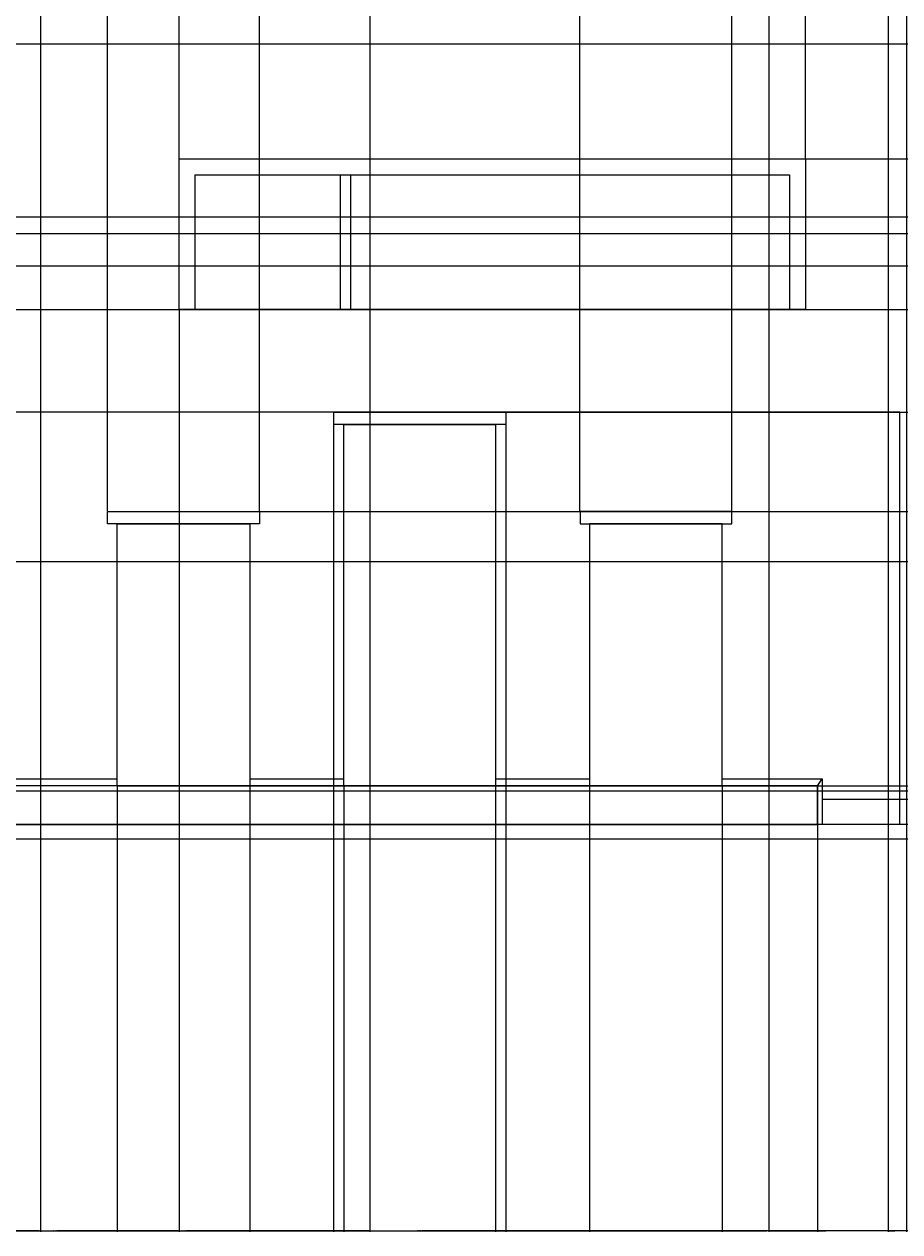
# Model space of a CAD drawing. Units: feet. Extents: x 2193 to 3502, y 890 to 1601.
# Tile 10 of 17: x 3145 to 3280, y 890 to 1076. Entities that reach past the tile are written whole.
import ezdxf

# ---------------------------------------------------------------- set-up
doc = ezdxf.new("R2010")
doc.units = ezdxf.units.FT
doc.layers.add('A-ANNO-DIMS', color=2, linetype='Continuous', lineweight=18)
doc.layers.add('A-ELEV', color=7, linetype='Continuous', lineweight=25)
doc.styles.get("Standard").update_dxf_attribs({"font": 'arial.ttf'})
doc.dimstyles.get("Standard").update_dxf_attribs({"dimtxt": 0.18, "dimasz": 0.18, "dimexe": 0.18, "dimexo": 0.0625, "dimgap": 0.09, "dimtad": 0, "dimtih": 1, "dimtoh": 1, "dimdec": 0, "dimzin": 0, "dimdsep": 46, "dimlunit": 3, "dimtxsty": 'Standard', "dimcen": 0.09, "dimadec": 0, "dimazin": 0, "dimtfac": 1, "dimtdec": 0, "dimtofl": 0, "dimtmove": 0, "dimatfit": 3, "dimfxl": 1, "dimtolj": 1, "dimtzin": 0, "dimarcsym": 0})

# ---------------------------------------------------------------- blocks, each defined once
blk = doc.blocks.new('*D13')
at = {"layer": 'A-ANNO-DIMS', "color": 0, "lineweight": -2, "transparency": 16777216}
for p, q in [((2934.37, 950.89), (2934.37, 1601.47)), ((2934.55, 1601.29), (3186.64, 1601.29)), ((3439.51, 1601.29), (3187.43, 1601.29)), ((3439.69, 1541.11), (3439.69, 1601.47))]:
    blk.add_line(p, q, dxfattribs=at)
at = {"layer": 'A-ANNO-DIMS', "color": 0, "transparency": 16777216}
for points in [[(2934.55, 1601.32), (2934.55, 1601.26), (2934.37, 1601.29)], [(3439.51, 1601.32), (3439.51, 1601.26), (3439.69, 1601.29)]]:
    blk.add_solid(points, dxfattribs=at)
at = {"layer": 'Defpoints', "color": 0, "transparency": 16777216}
for p in [(3439.69, 1601.29), (3439.69, 1541.04), (2934.37, 950.82)]:
    blk.add_point(p, dxfattribs=at)
at = {"layer": 'A-ANNO-DIMS', "color": 0, "transparency": 16777216, "insert": (3187.03, 1601.29), "char_height": 0.18, "attachment_point": 5}
blk.add_mtext('\\A1;505.3', dxfattribs=at)
blk = doc.blocks.new('*D16')
at = {"layer": 'A-ANNO-DIMS', "color": 0, "lineweight": -2, "transparency": 16777216}
for p, q in [((3132, 956.87), (3132, 890.39)), ((3305.41, 950.76), (3305.41, 890.39)), ((3132.18, 890.57), (3218.32, 890.57)), ((3305.23, 890.57), (3219.09, 890.57))]:
    blk.add_line(p, q, dxfattribs=at)
at = {"layer": 'A-ANNO-DIMS', "color": 0, "transparency": 16777216}
for points in [[(3132.18, 890.6), (3132.18, 890.54), (3132, 890.57)], [(3305.23, 890.6), (3305.23, 890.54), (3305.41, 890.57)]]:
    blk.add_solid(points, dxfattribs=at)
at = {"layer": 'Defpoints', "color": 0, "transparency": 16777216}
for p in [(3132, 956.94), (3305.41, 950.82), (3305.41, 890.57)]:
    blk.add_point(p, dxfattribs=at)
at = {"layer": 'A-ANNO-DIMS', "color": 0, "transparency": 16777216, "insert": (3218.71, 890.57), "char_height": 0.18, "attachment_point": 5}
blk.add_mtext('\\A1;173.4', dxfattribs=at)
blk = doc.blocks.new('*D25')
at = {"layer": 'A-ANNO-DIMS', "color": 0, "lineweight": -2, "transparency": 16777216}
for p, q in [((3070.17, 1073.03), (3501.85, 1073.03)), ((3501.67, 1072.85), (3501.67, 1056.13)), ((3501.67, 1039.05), (3501.67, 1055.77)), ((3067.73, 1038.87), (3501.85, 1038.87))]:
    blk.add_line(p, q, dxfattribs=at)
at = {"layer": 'A-ANNO-DIMS', "color": 0, "transparency": 16777216}
for points in [[(3501.64, 1072.85), (3501.7, 1072.85), (3501.67, 1073.03)], [(3501.64, 1039.05), (3501.7, 1039.05), (3501.67, 1038.87)]]:
    blk.add_solid(points, dxfattribs=at)
at = {"layer": 'Defpoints', "color": 0, "transparency": 16777216}
for p in [(3070.11, 1073.03), (3501.67, 1073.03), (3067.66, 1038.87)]:
    blk.add_point(p, dxfattribs=at)
at = {"layer": 'A-ANNO-DIMS', "color": 0, "transparency": 16777216, "insert": (3501.67, 1055.95), "char_height": 0.18, "attachment_point": 5}
blk.add_mtext('\\A1;34.165', dxfattribs=at)
blk = doc.blocks.new('*D31')
at = {"layer": 'A-ANNO-DIMS', "color": 0, "lineweight": -2, "transparency": 16777216}
for p, q in [((2760.54, 1541.04), (3501.85, 1541.04)), ((3501.67, 1540.86), (3501.67, 1246.12)), ((3501.67, 951), (3501.67, 1245.75)), ((2762.27, 950.82), (3501.85, 950.82))]:
    blk.add_line(p, q, dxfattribs=at)
at = {"layer": 'A-ANNO-DIMS', "color": 0, "transparency": 16777216}
for points in [[(3501.64, 1540.86), (3501.7, 1540.86), (3501.67, 1541.04)], [(3501.64, 951), (3501.7, 951), (3501.67, 950.82)]]:
    blk.add_solid(points, dxfattribs=at)
at = {"layer": 'Defpoints', "color": 0, "transparency": 16777216}
for p in [(2760.47, 1541.04), (3501.67, 1541.04), (2762.2, 950.82)]:
    blk.add_point(p, dxfattribs=at)
at = {"layer": 'A-ANNO-DIMS', "color": 0, "transparency": 16777216, "insert": (3501.67, 1245.93), "char_height": 0.18, "attachment_point": 5}
blk.add_mtext('\\A1;590.2', dxfattribs=at)
blk = doc.blocks.new('*D61')
at = {"layer": 'A-ANNO-DIMS', "color": 0, "lineweight": -2, "transparency": 16777216}
for p, q in [((2974.12, 1078.97), (2974.12, 890.39)), ((3147.5, 1078.97), (3147.5, 890.39)), ((2974.3, 890.57), (3060.42, 890.57)), ((3147.32, 890.57), (3061.19, 890.57))]:
    blk.add_line(p, q, dxfattribs=at)
at = {"layer": 'A-ANNO-DIMS', "color": 0, "transparency": 16777216}
for points in [[(2974.3, 890.6), (2974.3, 890.54), (2974.12, 890.57)], [(3147.32, 890.6), (3147.32, 890.54), (3147.5, 890.57)]]:
    blk.add_solid(points, dxfattribs=at)
at = {"layer": 'Defpoints', "color": 0, "transparency": 16777216}
for p in [(2974.12, 1079.03), (3147.5, 1079.03), (3147.5, 890.57)]:
    blk.add_point(p, dxfattribs=at)
at = {"layer": 'A-ANNO-DIMS', "color": 0, "transparency": 16777216, "insert": (3060.81, 890.57), "char_height": 0.18, "attachment_point": 5}
blk.add_mtext('\\A1;173.4', dxfattribs=at)
blk = doc.blocks.new('*D80')
at = {"layer": 'A-ANNO-DIMS', "color": 0, "lineweight": -2, "transparency": 16777216}
for p, q in [((3198.15, 1233.5), (3198.15, 890.39)), ((3315.74, 1233.5), (3315.74, 890.39)), ((3198.33, 890.57), (3256.49, 890.57)), ((3315.56, 890.57), (3257.4, 890.57))]:
    blk.add_line(p, q, dxfattribs=at)
at = {"layer": 'A-ANNO-DIMS', "color": 0, "transparency": 16777216}
for points in [[(3198.33, 890.6), (3198.33, 890.54), (3198.15, 890.57)], [(3315.56, 890.6), (3315.56, 890.54), (3315.74, 890.57)]]:
    blk.add_solid(points, dxfattribs=at)
at = {"layer": 'Defpoints', "color": 0, "transparency": 16777216}
for p in [(3198.15, 1233.56), (3315.74, 1233.56), (3315.74, 890.57)]:
    blk.add_point(p, dxfattribs=at)
at = {"layer": 'A-ANNO-DIMS', "color": 0, "transparency": 16777216, "insert": (3256.94, 890.57), "char_height": 0.18, "attachment_point": 5}
blk.add_mtext('\\A1;117.58', dxfattribs=at)
blk = doc.blocks.new('*D83')
at = {"layer": 'A-ANNO-DIMS', "color": 0, "lineweight": -2, "transparency": 16777216}
for p, q in [((3147.5, 1133.05), (3147.5, 890.39)), ((3198.15, 1133.05), (3198.15, 890.39)), ((3147.68, 890.57), (3172.43, 890.57)), ((3197.97, 890.57), (3173.22, 890.57))]:
    blk.add_line(p, q, dxfattribs=at)
at = {"layer": 'A-ANNO-DIMS', "color": 0, "transparency": 16777216}
for points in [[(3147.68, 890.6), (3147.68, 890.54), (3147.5, 890.57)], [(3197.97, 890.6), (3197.97, 890.54), (3198.15, 890.57)]]:
    blk.add_solid(points, dxfattribs=at)
at = {"layer": 'Defpoints', "color": 0, "transparency": 16777216}
for p in [(3147.5, 1133.11), (3198.15, 1133.11), (3198.15, 890.57)]:
    blk.add_point(p, dxfattribs=at)
at = {"layer": 'A-ANNO-DIMS', "color": 0, "transparency": 16777216, "insert": (3172.83, 890.57), "char_height": 0.18, "attachment_point": 5}
blk.add_mtext('\\A1;50.65', dxfattribs=at)
blk = doc.blocks.new('*D85')
at = {"layer": 'A-ANNO-DIMS', "color": 0, "lineweight": -2, "transparency": 16777216}
for p, q in [((3259.46, 1133.05), (3259.46, 890.39)), ((3277.81, 1115.17), (3277.81, 890.39)), ((3259.64, 890.57), (3268.25, 890.57)), ((3277.63, 890.57), (3269.02, 890.57))]:
    blk.add_line(p, q, dxfattribs=at)
at = {"layer": 'A-ANNO-DIMS', "color": 0, "transparency": 16777216}
for points in [[(3259.64, 890.6), (3259.64, 890.54), (3259.46, 890.57)], [(3277.63, 890.6), (3277.63, 890.54), (3277.81, 890.57)]]:
    blk.add_solid(points, dxfattribs=at)
at = {"layer": 'Defpoints', "color": 0, "transparency": 16777216}
for p in [(3259.46, 1133.11), (3277.81, 1115.23), (3277.81, 890.57)]:
    blk.add_point(p, dxfattribs=at)
at = {"layer": 'A-ANNO-DIMS', "color": 0, "transparency": 16777216, "insert": (3268.63, 890.57), "char_height": 0.18, "attachment_point": 5}
blk.add_mtext('\\A1;18.35', dxfattribs=at)
blk = doc.blocks.new('*D86')
at = {"layer": 'A-ANNO-DIMS', "color": 0, "lineweight": -2, "transparency": 16777216}
for p, q in [((3277.81, 1115.17), (3277.81, 890.39)), ((3280.64, 1112.39), (3280.64, 890.39)), ((3277.99, 890.57), (3278.83, 890.57)), ((3280.46, 890.57), (3279.62, 890.57))]:
    blk.add_line(p, q, dxfattribs=at)
at = {"layer": 'A-ANNO-DIMS', "color": 0, "transparency": 16777216}
for points in [[(3277.99, 890.6), (3277.99, 890.54), (3277.81, 890.57)], [(3280.46, 890.6), (3280.46, 890.54), (3280.64, 890.57)]]:
    blk.add_solid(points, dxfattribs=at)
at = {"layer": 'Defpoints', "color": 0, "transparency": 16777216}
for p in [(3277.81, 1115.23), (3280.64, 1112.45), (3280.64, 890.57)]:
    blk.add_point(p, dxfattribs=at)
at = {"layer": 'A-ANNO-DIMS', "color": 0, "transparency": 16777216, "insert": (3279.22, 890.57), "char_height": 0.18, "attachment_point": 5}
blk.add_mtext('\\A1;2.832', dxfattribs=at)
blk = doc.blocks.new('*D97')
at = {"layer": 'A-ANNO-DIMS', "color": 0, "lineweight": -2, "transparency": 16777216}
for p, q in [((3111.13, 1032.26), (3111.13, 1601.47)), ((3111.31, 1601.29), (3207.6, 1601.29)), ((3304.79, 1601.29), (3208.51, 1601.29)), ((3304.97, 1032.26), (3304.97, 1601.47))]:
    blk.add_line(p, q, dxfattribs=at)
at = {"layer": 'A-ANNO-DIMS', "color": 0, "transparency": 16777216}
for points in [[(3111.31, 1601.32), (3111.31, 1601.26), (3111.13, 1601.29)], [(3304.79, 1601.32), (3304.79, 1601.26), (3304.97, 1601.29)]]:
    blk.add_solid(points, dxfattribs=at)
at = {"layer": 'Defpoints', "color": 0, "transparency": 16777216}
for p in [(3304.97, 1601.29), (3111.13, 1032.19), (3304.97, 1032.19)]:
    blk.add_point(p, dxfattribs=at)
at = {"layer": 'A-ANNO-DIMS', "color": 0, "transparency": 16777216, "insert": (3208.05, 1601.29), "char_height": 0.18, "attachment_point": 5}
blk.add_mtext('\\A1;193.84', dxfattribs=at)
blk = doc.blocks.new('*D100')
at = {"layer": 'A-ANNO-DIMS', "color": 0, "lineweight": -2, "transparency": 16777216}
for p, q in [((3168.83, 1055.37), (3168.83, 1601.47)), ((3169.01, 1601.29), (3216.57, 1601.29)), ((3264.92, 1601.29), (3217.36, 1601.29)), ((3265.1, 1055.37), (3265.1, 1601.47))]:
    blk.add_line(p, q, dxfattribs=at)
at = {"layer": 'A-ANNO-DIMS', "color": 0, "transparency": 16777216}
for points in [[(3169.01, 1601.32), (3169.01, 1601.26), (3168.83, 1601.29)], [(3264.92, 1601.32), (3264.92, 1601.26), (3265.1, 1601.29)]]:
    blk.add_solid(points, dxfattribs=at)
at = {"layer": 'Defpoints', "color": 0, "transparency": 16777216}
for p in [(3265.1, 1601.29), (3168.83, 1055.31), (3265.1, 1055.31)]:
    blk.add_point(p, dxfattribs=at)
at = {"layer": 'A-ANNO-DIMS', "color": 0, "transparency": 16777216, "insert": (3216.97, 1601.29), "char_height": 0.18, "attachment_point": 5}
blk.add_mtext('\\A1;96.27', dxfattribs=at)
blk = doc.blocks.new('*D101')
at = {"layer": 'A-ANNO-DIMS', "color": 0, "lineweight": -2, "transparency": 16777216}
for p, q in [((3265.16, 1055.31), (3501.85, 1055.31)), ((3501.67, 1055.13), (3501.67, 1043.93)), ((3501.67, 1032.37), (3501.67, 1043.57)), ((3265.16, 1032.19), (3501.85, 1032.19))]:
    blk.add_line(p, q, dxfattribs=at)
at = {"layer": 'A-ANNO-DIMS', "color": 0, "transparency": 16777216}
for points in [[(3501.64, 1055.13), (3501.7, 1055.13), (3501.67, 1055.31)], [(3501.64, 1032.37), (3501.7, 1032.37), (3501.67, 1032.19)]]:
    blk.add_solid(points, dxfattribs=at)
at = {"layer": 'Defpoints', "color": 0, "transparency": 16777216}
for p in [(3265.1, 1055.31), (3501.67, 1055.31), (3265.1, 1032.19)]:
    blk.add_point(p, dxfattribs=at)
at = {"layer": 'A-ANNO-DIMS', "color": 0, "transparency": 16777216, "insert": (3501.67, 1043.75), "char_height": 0.18, "attachment_point": 5}
blk.add_mtext('\\A1;23.113', dxfattribs=at)
blk = doc.blocks.new('*D102')
at = {"layer": 'A-ANNO-DIMS', "color": 0, "lineweight": -2, "transparency": 16777216}
for p, q in [((3132, 1032.13), (3132, 890.39)), ((3168.83, 1032.13), (3168.83, 890.39)), ((3132.18, 890.57), (3149.95, 890.57)), ((3168.65, 890.57), (3150.88, 890.57))]:
    blk.add_line(p, q, dxfattribs=at)
at = {"layer": 'A-ANNO-DIMS', "color": 0, "transparency": 16777216}
for points in [[(3132.18, 890.6), (3132.18, 890.54), (3132, 890.57)], [(3168.65, 890.6), (3168.65, 890.54), (3168.83, 890.57)]]:
    blk.add_solid(points, dxfattribs=at)
at = {"layer": 'Defpoints', "color": 0, "transparency": 16777216}
for p in [(3132, 1032.19), (3168.83, 1032.19), (3168.83, 890.57)]:
    blk.add_point(p, dxfattribs=at)
at = {"layer": 'A-ANNO-DIMS', "color": 0, "transparency": 16777216, "insert": (3150.42, 890.57), "char_height": 0.18, "attachment_point": 5}
blk.add_mtext('\\A1;36.835', dxfattribs=at)
blk = doc.blocks.new('*D104')
at = {"layer": 'A-ANNO-DIMS', "color": 0, "lineweight": -2, "transparency": 16777216}
for p, q in [((3157.83, 1001.2), (3157.83, 1601.47)), ((3158.01, 1601.29), (3169.1, 1601.29)), ((3180.99, 1601.29), (3169.89, 1601.29)), ((3181.17, 1001.2), (3181.17, 1601.47))]:
    blk.add_line(p, q, dxfattribs=at)
at = {"layer": 'A-ANNO-DIMS', "color": 0, "transparency": 16777216}
for points in [[(3158.01, 1601.32), (3158.01, 1601.26), (3157.83, 1601.29)], [(3180.99, 1601.32), (3180.99, 1601.26), (3181.17, 1601.29)]]:
    blk.add_solid(points, dxfattribs=at)
at = {"layer": 'Defpoints', "color": 0, "transparency": 16777216}
for p in [(3181.17, 1601.29), (3157.83, 1001.13), (3181.17, 1001.13)]:
    blk.add_point(p, dxfattribs=at)
at = {"layer": 'A-ANNO-DIMS', "color": 0, "transparency": 16777216, "insert": (3169.5, 1601.29), "char_height": 0.18, "attachment_point": 5}
blk.add_mtext('\\A1;23.34', dxfattribs=at)
blk = doc.blocks.new('*D105')
at = {"layer": 'A-ANNO-DIMS', "color": 0, "lineweight": -2, "transparency": 16777216}
for p, q in [((3192.55, 1014.45), (3192.55, 890.39)), ((3219.06, 1014.45), (3219.06, 890.39)), ((3192.73, 890.57), (3205.34, 890.57)), ((3218.88, 890.57), (3206.27, 890.57))]:
    blk.add_line(p, q, dxfattribs=at)
at = {"layer": 'A-ANNO-DIMS', "color": 0, "transparency": 16777216}
for points in [[(3192.73, 890.6), (3192.73, 890.54), (3192.55, 890.57)], [(3218.88, 890.6), (3218.88, 890.54), (3219.06, 890.57)]]:
    blk.add_solid(points, dxfattribs=at)
at = {"layer": 'Defpoints', "color": 0, "transparency": 16777216}
for p in [(3192.55, 1014.51), (3219.06, 1014.51), (3219.06, 890.57)]:
    blk.add_point(p, dxfattribs=at)
at = {"layer": 'A-ANNO-DIMS', "color": 0, "transparency": 16777216, "insert": (3205.8, 890.57), "char_height": 0.18, "attachment_point": 5}
blk.add_mtext('\\A1;26.514', dxfattribs=at)
blk = doc.blocks.new('*D106')
at = {"layer": 'A-ANNO-DIMS', "color": 0, "lineweight": -2, "transparency": 16777216}
for p, q in [((3230.44, 1001.2), (3230.44, 1601.47)), ((3230.62, 1601.29), (3241.72, 1601.29)), ((3253.6, 1601.29), (3242.51, 1601.29)), ((3253.78, 1001.2), (3253.78, 1601.47))]:
    blk.add_line(p, q, dxfattribs=at)
at = {"layer": 'A-ANNO-DIMS', "color": 0, "transparency": 16777216}
for points in [[(3230.62, 1601.32), (3230.62, 1601.26), (3230.44, 1601.29)], [(3253.6, 1601.32), (3253.6, 1601.26), (3253.78, 1601.29)]]:
    blk.add_solid(points, dxfattribs=at)
at = {"layer": 'Defpoints', "color": 0, "transparency": 16777216}
for p in [(3253.78, 1601.29), (3230.44, 1001.13), (3253.78, 1001.13)]:
    blk.add_point(p, dxfattribs=at)
at = {"layer": 'A-ANNO-DIMS', "color": 0, "transparency": 16777216, "insert": (3242.11, 1601.29), "char_height": 0.18, "attachment_point": 5}
blk.add_mtext('\\A1;23.34', dxfattribs=at)
blk = doc.blocks.new('*D107')
at = {"layer": 'A-ANNO-DIMS', "color": 0, "lineweight": -2, "transparency": 16777216}
for p, q in [((3140.22, 958.89), (3140.22, 890.39)), ((3159.3, 958.89), (3159.3, 890.39)), ((3140.4, 890.57), (3149.3, 890.57)), ((3159.12, 890.57), (3150.22, 890.57))]:
    blk.add_line(p, q, dxfattribs=at)
at = {"layer": 'A-ANNO-DIMS', "color": 0, "transparency": 16777216}
for points in [[(3140.4, 890.6), (3140.4, 890.54), (3140.22, 890.57)], [(3159.12, 890.6), (3159.12, 890.54), (3159.3, 890.57)]]:
    blk.add_solid(points, dxfattribs=at)
at = {"layer": 'Defpoints', "color": 0, "transparency": 16777216}
for p in [(3140.22, 958.96), (3159.3, 958.96), (3159.3, 890.57)]:
    blk.add_point(p, dxfattribs=at)
at = {"layer": 'A-ANNO-DIMS', "color": 0, "transparency": 16777216, "insert": (3149.76, 890.57), "char_height": 0.18, "attachment_point": 5}
blk.add_mtext('\\A1;19.075', dxfattribs=at)
blk = doc.blocks.new('*D108')
at = {"layer": 'A-ANNO-DIMS', "color": 0, "lineweight": -2, "transparency": 16777216}
for p, q in [((3159.3, 958.89), (3159.3, 890.39)), ((3179.69, 958.89), (3179.69, 890.39)), ((3159.48, 890.57), (3169.03, 890.57)), ((3179.51, 890.57), (3169.96, 890.57))]:
    blk.add_line(p, q, dxfattribs=at)
at = {"layer": 'A-ANNO-DIMS', "color": 0, "transparency": 16777216}
for points in [[(3159.48, 890.6), (3159.48, 890.54), (3159.3, 890.57)], [(3179.51, 890.6), (3179.51, 890.54), (3179.69, 890.57)]]:
    blk.add_solid(points, dxfattribs=at)
at = {"layer": 'Defpoints', "color": 0, "transparency": 16777216}
for p in [(3159.3, 958.96), (3179.69, 958.96), (3179.69, 890.57)]:
    blk.add_point(p, dxfattribs=at)
at = {"layer": 'A-ANNO-DIMS', "color": 0, "transparency": 16777216, "insert": (3169.5, 890.57), "char_height": 0.18, "attachment_point": 5}
blk.add_mtext('\\A1;20.397', dxfattribs=at)
blk = doc.blocks.new('*D109')
at = {"layer": 'A-ANNO-DIMS', "color": 0, "lineweight": -2, "transparency": 16777216}
for p, q in [((3179.69, 958.89), (3179.69, 890.39)), ((3194.13, 958.89), (3194.13, 890.39)), ((3179.87, 890.57), (3186.53, 890.57)), ((3193.95, 890.57), (3187.3, 890.57))]:
    blk.add_line(p, q, dxfattribs=at)
at = {"layer": 'A-ANNO-DIMS', "color": 0, "transparency": 16777216}
for points in [[(3179.87, 890.6), (3179.87, 890.54), (3179.69, 890.57)], [(3193.95, 890.6), (3193.95, 890.54), (3194.13, 890.57)]]:
    blk.add_solid(points, dxfattribs=at)
at = {"layer": 'Defpoints', "color": 0, "transparency": 16777216}
for p in [(3179.69, 958.96), (3194.13, 958.96), (3194.13, 890.57)]:
    blk.add_point(p, dxfattribs=at)
at = {"layer": 'A-ANNO-DIMS', "color": 0, "transparency": 16777216, "insert": (3186.91, 890.57), "char_height": 0.18, "attachment_point": 5}
blk.add_mtext('\\A1;14.44', dxfattribs=at)
blk = doc.blocks.new('*D110')
at = {"layer": 'A-ANNO-DIMS', "color": 0, "lineweight": -2, "transparency": 16777216}
for p, q in [((3194.13, 958.89), (3194.13, 890.39)), ((3217.47, 958.89), (3217.47, 890.39)), ((3194.31, 890.57), (3205.41, 890.57)), ((3217.29, 890.57), (3206.2, 890.57))]:
    blk.add_line(p, q, dxfattribs=at)
at = {"layer": 'A-ANNO-DIMS', "color": 0, "transparency": 16777216}
for points in [[(3194.31, 890.6), (3194.31, 890.54), (3194.13, 890.57)], [(3217.29, 890.6), (3217.29, 890.54), (3217.47, 890.57)]]:
    blk.add_solid(points, dxfattribs=at)
at = {"layer": 'Defpoints', "color": 0, "transparency": 16777216}
for p in [(3194.13, 958.96), (3217.47, 958.96), (3217.47, 890.57)]:
    blk.add_point(p, dxfattribs=at)
at = {"layer": 'A-ANNO-DIMS', "color": 0, "transparency": 16777216, "insert": (3205.8, 890.57), "char_height": 0.18, "attachment_point": 5}
blk.add_mtext('\\A1;23.34', dxfattribs=at)
blk = doc.blocks.new('*D111')
at = {"layer": 'A-ANNO-DIMS', "color": 0, "lineweight": -2, "transparency": 16777216}
for p, q in [((3217.47, 958.89), (3217.47, 890.39)), ((3231.91, 958.89), (3231.91, 890.39)), ((3217.65, 890.57), (3224.31, 890.57)), ((3231.73, 890.57), (3225.08, 890.57))]:
    blk.add_line(p, q, dxfattribs=at)
at = {"layer": 'A-ANNO-DIMS', "color": 0, "transparency": 16777216}
for points in [[(3217.65, 890.6), (3217.65, 890.54), (3217.47, 890.57)], [(3231.73, 890.6), (3231.73, 890.54), (3231.91, 890.57)]]:
    blk.add_solid(points, dxfattribs=at)
at = {"layer": 'Defpoints', "color": 0, "transparency": 16777216}
for p in [(3217.47, 958.96), (3231.91, 958.96), (3231.91, 890.57)]:
    blk.add_point(p, dxfattribs=at)
at = {"layer": 'A-ANNO-DIMS', "color": 0, "transparency": 16777216, "insert": (3224.69, 890.57), "char_height": 0.18, "attachment_point": 5}
blk.add_mtext('\\A1;14.44', dxfattribs=at)
blk = doc.blocks.new('*D112')
at = {"layer": 'A-ANNO-DIMS', "color": 0, "lineweight": -2, "transparency": 16777216}
for p, q in [((3231.91, 958.89), (3231.91, 890.39)), ((3252.31, 958.89), (3252.31, 890.39)), ((3232.09, 890.57), (3241.65, 890.57)), ((3252.13, 890.57), (3242.58, 890.57))]:
    blk.add_line(p, q, dxfattribs=at)
at = {"layer": 'A-ANNO-DIMS', "color": 0, "transparency": 16777216}
for points in [[(3232.09, 890.6), (3232.09, 890.54), (3231.91, 890.57)], [(3252.13, 890.6), (3252.13, 890.54), (3252.31, 890.57)]]:
    blk.add_solid(points, dxfattribs=at)
at = {"layer": 'Defpoints', "color": 0, "transparency": 16777216}
for p in [(3231.91, 958.96), (3252.31, 958.96), (3252.31, 890.57)]:
    blk.add_point(p, dxfattribs=at)
at = {"layer": 'A-ANNO-DIMS', "color": 0, "transparency": 16777216, "insert": (3242.11, 890.57), "char_height": 0.18, "attachment_point": 5}
blk.add_mtext('\\A1;20.397', dxfattribs=at)
blk = doc.blocks.new('*D113')
at = {"layer": 'A-ANNO-DIMS', "color": 0, "lineweight": -2, "transparency": 16777216}
for p, q in [((3252.31, 958.89), (3252.31, 890.39)), ((3266.93, 958.89), (3266.93, 890.39)), ((3252.49, 890.57), (3259.16, 890.57)), ((3266.75, 890.57), (3260.07, 890.57))]:
    blk.add_line(p, q, dxfattribs=at)
at = {"layer": 'A-ANNO-DIMS', "color": 0, "transparency": 16777216}
for points in [[(3252.49, 890.6), (3252.49, 890.54), (3252.31, 890.57)], [(3266.75, 890.6), (3266.75, 890.54), (3266.93, 890.57)]]:
    blk.add_solid(points, dxfattribs=at)
at = {"layer": 'Defpoints', "color": 0, "transparency": 16777216}
for p in [(3252.31, 958.96), (3266.93, 958.96), (3266.93, 890.57)]:
    blk.add_point(p, dxfattribs=at)
at = {"layer": 'A-ANNO-DIMS', "color": 0, "transparency": 16777216, "insert": (3259.62, 890.57), "char_height": 0.18, "attachment_point": 5}
blk.add_mtext('\\A1;14.615', dxfattribs=at)
blk = doc.blocks.new('*D114')
at = {"layer": 'A-ANNO-DIMS', "color": 0, "lineweight": -2, "transparency": 16777216}
for p, q in [((3157.89, 1001.13), (3501.85, 1001.13)), ((3501.67, 1000.95), (3501.67, 980.23)), ((3501.67, 959.14), (3501.67, 979.86)), ((3159.36, 958.96), (3501.85, 958.96))]:
    blk.add_line(p, q, dxfattribs=at)
at = {"layer": 'A-ANNO-DIMS', "color": 0, "transparency": 16777216}
for points in [[(3501.64, 1000.95), (3501.7, 1000.95), (3501.67, 1001.13)], [(3501.64, 959.14), (3501.7, 959.14), (3501.67, 958.96)]]:
    blk.add_solid(points, dxfattribs=at)
at = {"layer": 'Defpoints', "color": 0, "transparency": 16777216}
for p in [(3157.83, 1001.13), (3501.67, 1001.13), (3159.3, 958.96)]:
    blk.add_point(p, dxfattribs=at)
at = {"layer": 'A-ANNO-DIMS', "color": 0, "transparency": 16777216, "insert": (3501.67, 980.04), "char_height": 0.18, "attachment_point": 5}
blk.add_mtext('\\A1;42.18', dxfattribs=at)
blk = doc.blocks.new('*D115')
at = {"layer": 'A-ANNO-DIMS', "color": 0, "lineweight": -2, "transparency": 16777216}
for p, q in [((3192.61, 1016.4), (3501.85, 1016.4)), ((3501.67, 1016.22), (3501.67, 987.86)), ((3501.67, 959.14), (3501.67, 987.5)), ((3194.2, 958.96), (3501.85, 958.96))]:
    blk.add_line(p, q, dxfattribs=at)
at = {"layer": 'A-ANNO-DIMS', "color": 0, "transparency": 16777216}
for points in [[(3501.64, 1016.22), (3501.7, 1016.22), (3501.67, 1016.4)], [(3501.64, 959.14), (3501.7, 959.14), (3501.67, 958.96)]]:
    blk.add_solid(points, dxfattribs=at)
at = {"layer": 'Defpoints', "color": 0, "transparency": 16777216}
for p in [(3192.55, 1016.4), (3501.67, 1016.4), (3194.13, 958.96)]:
    blk.add_point(p, dxfattribs=at)
at = {"layer": 'A-ANNO-DIMS', "color": 0, "transparency": 16777216, "insert": (3501.67, 987.68), "char_height": 0.18, "attachment_point": 5}
blk.add_mtext('\\A1;57.44', dxfattribs=at)
blk = doc.blocks.new('*D124')
at = {"layer": 'A-ANNO-DIMS', "color": 0, "lineweight": -2, "transparency": 16777216}
for p, q in [((3304.91, 1046.36), (2193.56, 1046.36)), ((2193.74, 1046.18), (2193.74, 1045.26)), ((3304.91, 1043.78), (2193.56, 1043.78)), ((2193.74, 1043.96), (2193.74, 1044.89))]:
    blk.add_line(p, q, dxfattribs=at)
at = {"layer": 'A-ANNO-DIMS', "color": 0, "transparency": 16777216}
for points in [[(2193.71, 1046.18), (2193.77, 1046.18), (2193.74, 1046.36)], [(2193.71, 1043.96), (2193.77, 1043.96), (2193.74, 1043.78)]]:
    blk.add_solid(points, dxfattribs=at)
at = {"layer": 'Defpoints', "color": 0, "transparency": 16777216}
for p in [(3304.97, 1046.36), (2193.74, 1043.78), (3304.97, 1043.78)]:
    blk.add_point(p, dxfattribs=at)
at = {"layer": 'A-ANNO-DIMS', "color": 0, "transparency": 16777216, "insert": (2193.74, 1045.07), "char_height": 0.18, "attachment_point": 5}
blk.add_mtext('\\A1;2.583', dxfattribs=at)
blk = doc.blocks.new('*D130')
at = {"layer": 'A-ANNO-DIMS', "color": 0, "lineweight": -2, "transparency": 16777216}
for p, q in [((3304.91, 993.39), (2193.56, 993.39)), ((2193.74, 993.21), (2193.74, 975.95)), ((2193.74, 958.33), (2193.74, 975.59)), ((3304.91, 958.15), (2193.56, 958.15))]:
    blk.add_line(p, q, dxfattribs=at)
at = {"layer": 'A-ANNO-DIMS', "color": 0, "transparency": 16777216}
for points in [[(2193.71, 993.21), (2193.77, 993.21), (2193.74, 993.39)], [(2193.71, 958.33), (2193.77, 958.33), (2193.74, 958.15)]]:
    blk.add_solid(points, dxfattribs=at)
at = {"layer": 'Defpoints', "color": 0, "transparency": 16777216}
for p in [(2193.74, 993.39), (3304.97, 993.39), (3304.97, 958.15)]:
    blk.add_point(p, dxfattribs=at)
at = {"layer": 'A-ANNO-DIMS', "color": 0, "transparency": 16777216, "insert": (2193.74, 975.77), "char_height": 0.18, "attachment_point": 5}
blk.add_mtext('\\A1;35.24', dxfattribs=at)

msp = doc.modelspace()

# ---------------------------------------------------------------- linework, layer by layer
at = {"layer": 'A-ELEV'}
for p, q in [((2934.3742, 1073.031), (3439.6901, 1073.031)), ((3192.5464, 1016.4), (3192.5464, 1014.5106)), ((3219.0609, 1016.4), (3219.0609, 1014.5106)), ((3142.4884, 960.0129), (3159.2977, 960.0129)), ((3179.6947, 960.0129), (3194.1338, 960.0129)), ((3217.4736, 960.0129), (3231.9126, 960.0129)), ((3252.3096, 960.0129), (3267.6446, 960.0129)), ((3266.9251, 958.9555), (3267.6446, 960.0129)), ((3267.6446, 960.0129), (3267.6446, 953.031)), ((3267.6446, 956.8829), (3304.9731, 956.8829))]:
    msp.add_line(p, q, dxfattribs=at)
for points in [[(3265.1012, 1032.1935), (3168.8336, 1032.1935), (3168.8336, 1055.3069), (3265.1012, 1055.3069)], [(3193.646, 1052.8618), (3195.1383, 1052.8618), (3195.1383, 1032.1935), (3193.646, 1032.1935)], [(3181.1661, 999.2439), (3157.8263, 999.2439), (3157.8263, 1001.1334), (3181.1661, 1001.1334)], [(3230.4412, 999.2439), (3253.781, 999.2439), (3253.781, 1001.1334), (3230.4412, 1001.1334)], [(3140.2223, 953.031), (3266.9251, 953.031), (3266.9251, 958.9555), (3140.2223, 958.9555)], [(2934.3742, 950.8228), (3305.4139, 950.8228), (3305.4139, 953.031), (2934.3742, 953.031)]]:
    msp.add_lwpolyline(points, close=True, dxfattribs=at)
for points in [[(3171.2788, 1032.1935), (3171.2788, 1052.8618), (3262.6561, 1052.8618), (3262.6561, 1032.1935)], [(3111.1302, 1016.4), (3111.1302, 1032.1935), (3304.9731, 1032.1935), (3304.9731, 956.8829)], [(3279.6085, 953.031), (3279.6085, 1016.4), (3111.1302, 1016.4)], [(3192.5464, 1016.4), (3219.0609, 1016.4)], [(3219.0609, 1014.5106), (3192.5464, 1014.5106)], [(3194.1338, 958.9555), (3194.1338, 1014.5106), (3217.4736, 1014.5106), (3217.4736, 958.9555)], [(3159.2977, 958.9555), (3159.2977, 999.2439), (3179.6947, 999.2439), (3179.6947, 958.9555)], [(3252.3096, 958.9555), (3252.3096, 999.2439), (3231.9126, 999.2439), (3231.9126, 958.9555)]]:
    msp.add_lwpolyline(points, dxfattribs=at)

# ---------------------------------------------------------------- dimensions: what is measured, and where the dimension line sits
at = {"layer": 'A-ANNO-DIMS'}
for base, p1, p2, override, picture, middle in [((3439.6901, 1601.2941), (2934.3742, 950.8228), (3439.6901, 1541.0441), {"dimdec": 1, "dimlfac": 1, "dimrnd": 0, "dimzin": 0, "dimdsep": 46, "dimlunit": 2}, '*D13', (3187.0321, 1601.2941)), ((3304.9731, 1601.2941), (3111.1302, 1032.1935), (3304.9731, 1032.1935), {"dimdec": 2, "dimlfac": 1, "dimrnd": 0, "dimzin": 0, "dimdsep": 46, "dimlunit": 2}, '*D97', (3208.0516, 1601.2941)), ((3181.1661, 1601.2941), (3157.8263, 1001.1334), (3181.1661, 1001.1334), {"dimdec": 2, "dimlfac": 1, "dimrnd": 0, "dimzin": 0, "dimdsep": 46, "dimlunit": 2}, '*D104', (3169.4962, 1601.2941)), ((3265.1012, 1601.2941), (3168.8336, 1055.3069), (3265.1012, 1055.3069), {"dimdec": 2, "dimlfac": 1, "dimrnd": 0, "dimzin": 0, "dimdsep": 46, "dimlunit": 2}, '*D100', (3216.9674, 1601.2941)), ((3253.781, 1601.2941), (3230.4412, 1001.1334), (3253.781, 1001.1334), {"dimdec": 2, "dimlfac": 1, "dimrnd": 0, "dimzin": 0, "dimdsep": 46, "dimlunit": 2}, '*D106', (3242.1111, 1601.2941)), ((3315.7352, 890.5728), (3198.1547, 1233.561), (3315.7352, 1233.561), {"dimdec": 2, "dimlfac": 1, "dimrnd": 0, "dimzin": 0, "dimdsep": 46, "dimlunit": 2}, '*D80', (3256.9449, 890.5728)), ((3198.1547, 890.5728), (3147.5022, 1133.1128), (3198.1547, 1133.1128), {"dimdec": 2, "dimlfac": 1, "dimrnd": 0, "dimzin": 0, "dimdsep": 46, "dimlunit": 2}, '*D83', (3172.8284, 890.5728)), ((3277.8077, 890.5728), (3259.4585, 1133.1128), (3277.8077, 1115.2331), {"dimdec": 2, "dimlfac": 1, "dimrnd": 0, "dimzin": 0, "dimdsep": 46, "dimlunit": 2}, '*D85', (3268.6331, 890.5728)), ((3280.6398, 890.5728), (3277.8077, 1115.2331), (3280.6398, 1112.4498), {"dimdec": 3, "dimlfac": 1, "dimrnd": 0, "dimzin": 0, "dimdsep": 46, "dimlunit": 2}, '*D86', (3279.2237, 890.5728)), ((3147.5022, 890.5728), (2974.116, 1079.031), (3147.5022, 1079.031), {"dimdec": 1, "dimlfac": 1, "dimrnd": 0, "dimzin": 0, "dimdsep": 46, "dimlunit": 2}, '*D61', (3060.8091, 890.5728)), ((3168.8336, 890.5728), (3131.9988, 1032.1935), (3168.8336, 1032.1935), {"dimdec": 3, "dimlfac": 1, "dimrnd": 0, "dimzin": 0, "dimdsep": 46, "dimlunit": 2}, '*D102', (3150.4162, 890.5728)), ((3219.06089, 890.57279), (3192.54645, 1014.51056), (3219.06089, 1014.51056), {"dimdec": 3, "dimlfac": 1, "dimrnd": 0, "dimzin": 0, "dimdsep": 46, "dimlunit": 2}, '*D105', (3205.80367, 890.57279)), ((3159.2977, 890.5728), (3140.2223, 958.9555), (3159.2977, 958.9555), {"dimdec": 3, "dimlfac": 1, "dimrnd": 0, "dimzin": 0, "dimdsep": 46, "dimlunit": 2}, '*D107', (3149.76, 890.5728)), ((3179.6947, 890.5728), (3159.2977, 958.9555), (3179.6947, 958.9555), {"dimdec": 3, "dimlfac": 1, "dimrnd": 0, "dimzin": 0, "dimdsep": 46, "dimlunit": 2}, '*D108', (3169.4962, 890.5728)), ((3194.1338, 890.5728), (3179.6947, 958.9555), (3194.1338, 958.9555), {"dimdec": 2, "dimlfac": 1, "dimrnd": 0, "dimzin": 0, "dimdsep": 46, "dimlunit": 2}, '*D109', (3186.9142, 890.5728)), ((3217.4736, 890.5728), (3194.1338, 958.9555), (3217.4736, 958.9555), {"dimdec": 2, "dimlfac": 1, "dimrnd": 0, "dimzin": 0, "dimdsep": 46, "dimlunit": 2}, '*D110', (3205.8037, 890.5728)), ((3231.9126, 890.5728), (3217.4736, 958.9555), (3231.9126, 958.9555), {"dimdec": 2, "dimlfac": 1, "dimrnd": 0, "dimzin": 0, "dimdsep": 46, "dimlunit": 2}, '*D111', (3224.6931, 890.5728)), ((3252.3096, 890.5728), (3231.9126, 958.9555), (3252.3096, 958.9555), {"dimdec": 3, "dimlfac": 1, "dimrnd": 0, "dimzin": 0, "dimdsep": 46, "dimlunit": 2}, '*D112', (3242.1111, 890.5728)), ((3266.92514, 890.57279), (3252.309645, 958.955458), (3266.92514, 958.955458), {"dimdec": 3, "dimlfac": 1, "dimrnd": 0, "dimzin": 0, "dimdsep": 46, "dimlunit": 2}, '*D113', (3259.617392, 890.57279)), ((3305.4139, 890.5728), (3131.9988, 956.9371), (3305.4139, 950.8228), {"dimdec": 1, "dimlfac": 1, "dimrnd": 0, "dimzin": 0, "dimdsep": 46, "dimlunit": 2}, '*D16', (3218.7064, 890.5728))]:
    dim = msp.add_linear_dim(base=base, p1=p1, p2=p2, dimstyle='Standard', override=override, dxfattribs=at)
    dim.commit()
    dim.dimension.update_dxf_attribs({"geometry": picture, "text_midpoint": middle})
for base, p1, p2, override, picture, middle in [((3501.6716, 1541.0441), (2762.2048, 950.8228), (2760.4733, 1541.0441), {"dimdec": 1, "dimlfac": 1, "dimrnd": 0, "dimzin": 0, "dimdsep": 46, "dimlunit": 2}, '*D31', (3501.6716, 1245.9334)), ((3501.6716, 1073.031), (3067.665, 1038.8658), (3070.1101, 1073.031), {"dimdec": 3, "dimlfac": 1, "dimrnd": 0, "dimzin": 0, "dimdsep": 46, "dimlunit": 2}, '*D25', (3501.6716, 1055.9484)), ((3501.6716, 1055.3069), (3265.1012, 1032.1935), (3265.1012, 1055.3069), {"dimdec": 3, "dimlfac": 1, "dimrnd": 0, "dimzin": 0, "dimdsep": 46, "dimlunit": 2}, '*D101', (3501.6716, 1043.7502)), ((2193.7417, 1043.7821), (3304.9731, 1046.365), (3304.9731, 1043.7821), {"dimdec": 3, "dimlfac": 1, "dimrnd": 0, "dimzin": 0, "dimdsep": 46, "dimlunit": 2}, '*D124', (2193.7417, 1045.0735)), ((3501.6716, 1016.4), (3194.1338, 958.9555), (3192.5464, 1016.4), {"dimdec": 2, "dimlfac": 1, "dimrnd": 0, "dimzin": 0, "dimdsep": 46, "dimlunit": 2}, '*D115', (3501.6716, 987.6777)), ((3501.6716, 1001.1334), (3159.2977, 958.9555), (3157.8263, 1001.1334), {"dimdec": 2, "dimlfac": 1, "dimrnd": 0, "dimzin": 0, "dimdsep": 46, "dimlunit": 2}, '*D114', (3501.6716, 980.0444)), ((2193.7417, 993.3923), (3304.9731, 958.1519), (3304.9731, 993.3923), {"dimdec": 2, "dimlfac": 1, "dimrnd": 0, "dimzin": 0, "dimdsep": 46, "dimlunit": 2}, '*D130', (2193.7417, 975.7721))]:
    dim = msp.add_linear_dim(base=base, p1=p1, p2=p2, angle=90, dimstyle='Standard', override=override, dxfattribs=at)
    dim.commit()
    dim.dimension.update_dxf_attribs({"geometry": picture, "text_midpoint": middle})

doc.saveas('drawing.dxf')
